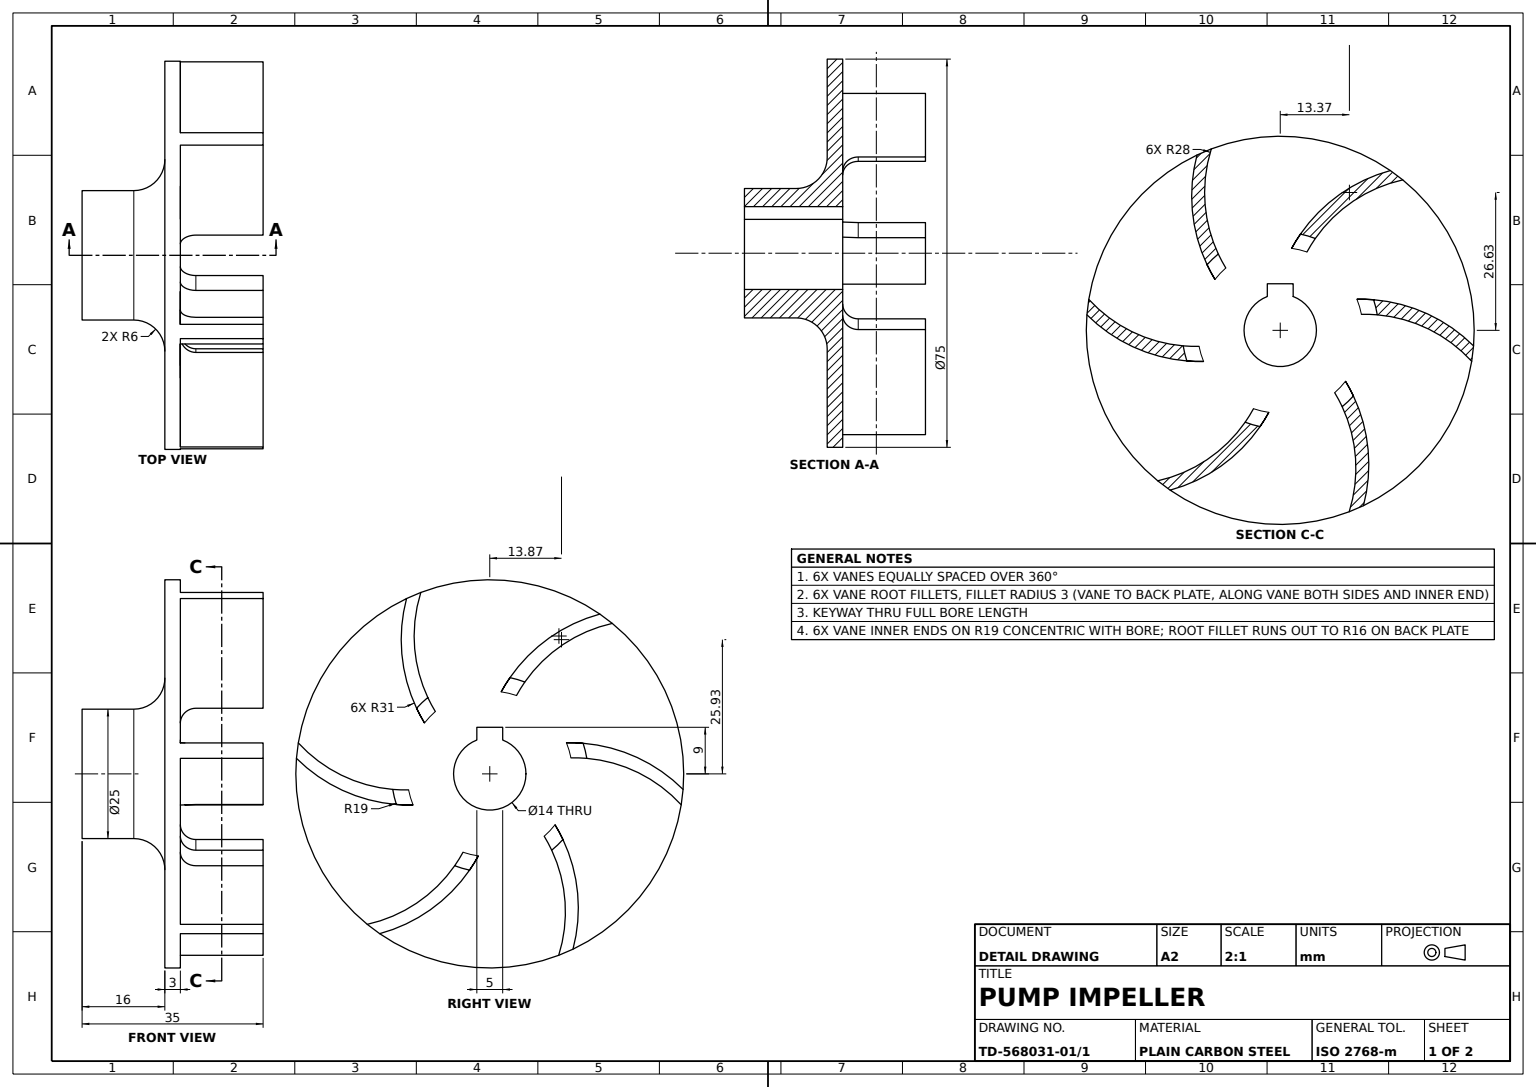
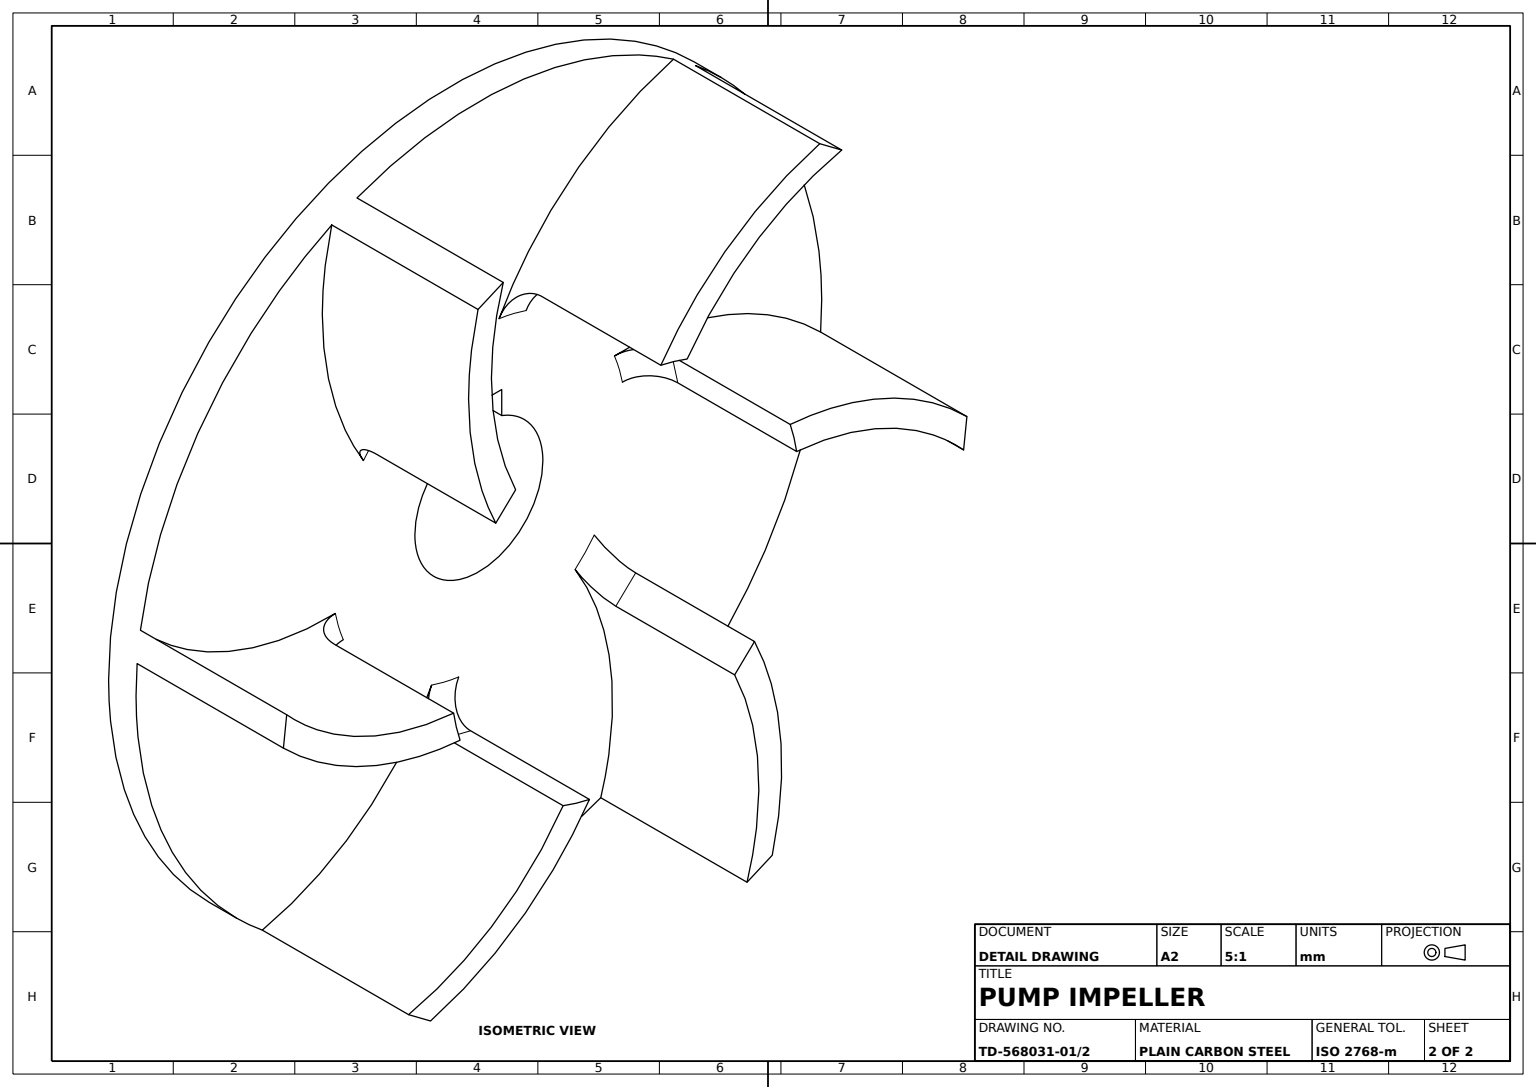
from build123d import *

# Parameters (mm, degrees)
BACK_PLATE_PROFILE_SKETCH_R              = 37.5
BACK_PLATE_75_DEPTH                      = 1.5
HUB_START                                = 16
HUB_SKETCH_25_R                          = 12.5
HUB_25_DEPTH                             = 16
HUB_ROOT_FILLET_R6_R                     = 6
VANE_DEPTH                               = 16
VANE_ROOT_FILLET_R3_R                    = 3
VANE_PATTERN_6X_COUNT                    = 6
VANE_ROOT_FILLET_R3_OF_VANE_PATTERN_6X_R = 3


with BuildPart() as part:
    # Back Plate Profile Sketch → Back Plate Ø75 (new, symmetric)
    with BuildSketch(Plane.XY):
        Circle(BACK_PLATE_PROFILE_SKETCH_R)
        with BuildLine():
            ThreePointArc((-2.5, 6.538348415), (0, -7), (2.5, 6.538348415))
            Line((2.5, 6.538348415), (2.5, 9))
            Line((2.5, 9), (-2.5, 9))
            Line((-2.5, 9), (-2.5, 6.538348415))
        make_face(mode=Mode.SUBTRACT)
    extrude(amount=BACK_PLATE_75_DEPTH, both=True)

    # Hub Sketch Ø25 → Hub Ø25 (add)
    with BuildSketch(Plane.XY.offset(1.5).offset(HUB_START)):
        Circle(HUB_SKETCH_25_R)
        with BuildLine():
            Line((2.5, 9), (2.5, 6.538348415))
            ThreePointArc((2.5, 6.538348415), (0, -7), (-2.5, 6.538348415))
            Line((-2.5, 6.538348415), (-2.5, 9))
            Line((-2.5, 9), (2.5, 9))
        make_face(mode=Mode.SUBTRACT)
    extrude(amount=-HUB_25_DEPTH)

    # Hub Root Fillet R6
    hub_root_fillet_r6_edges = [part.edges().sort_by_distance(p)[0] for p in [
        (-12.5, 0, 1.5),
    ]]
    fillet(hub_root_fillet_r6_edges, radius=HUB_ROOT_FILLET_R6_R)

    # Vane Profile Sketch → Vane (add)
    with BuildSketch(Plane(origin=(0, 0, -1.5), x_dir=(-1, 0, 0), z_dir=(0, 0, -1))):
        with BuildLine():
            ThreePointArc((-37.020384076, 5.978391325), (-28.735420007, -0.227993827), (-18.761663039, -3))
            ThreePointArc((-18.761663039, -3), (-18.46626176, -4.471820281), (-18.055586153, -5.915725541))
            ThreePointArc((-18.055586153, -5.915725541), (-28.50675968, -3.168102302), (-37.379807383, 3))
            ThreePointArc((-37.379807383, 3), (-37.229891566, 4.492791335), (-37.020384076, 5.978391325))
        make_face()
    vane = extrude(amount=VANE_DEPTH)

    # Vane Root Fillet R3
    vane_root_fillet_r3_edges = [part.edges().sort_by_distance(p)[0] for p in [
        (18.46626176, -4.471820281, -1.5),
    ]]
    fillet(vane_root_fillet_r3_edges, radius=VANE_ROOT_FILLET_R3_R)

    # Vane Pattern 6x: Vane ×6 about axis
    vane_pattern_6x_axis = Axis((0, 0, 0), (0, 0, 1))
    for i in range(1, VANE_PATTERN_6X_COUNT):
        add(vane.rotate(vane_pattern_6x_axis, i * 360 / VANE_PATTERN_6X_COUNT))

    # Vane Root Fillet R3 of Vane Pattern 6x
    vane_root_fillet_r3_of_vane_pattern_6x_edges = [part.edges().sort_by_distance(p)[0] for p in [
        (13.105840844, 13.756341656, -1.5),
        (-5.360420916, 18.228161937, -1.5),
        (-18.46626176, 4.471820281, -1.5),
        (-13.105840844, -13.756341656, -1.5),
        (5.360420916, -18.228161937, -1.5),
    ]]
    fillet(vane_root_fillet_r3_of_vane_pattern_6x_edges, radius=VANE_ROOT_FILLET_R3_OF_VANE_PATTERN_6X_R)


solid = part.part
